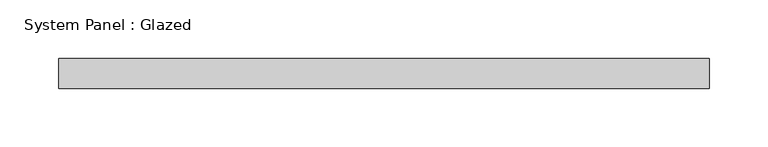
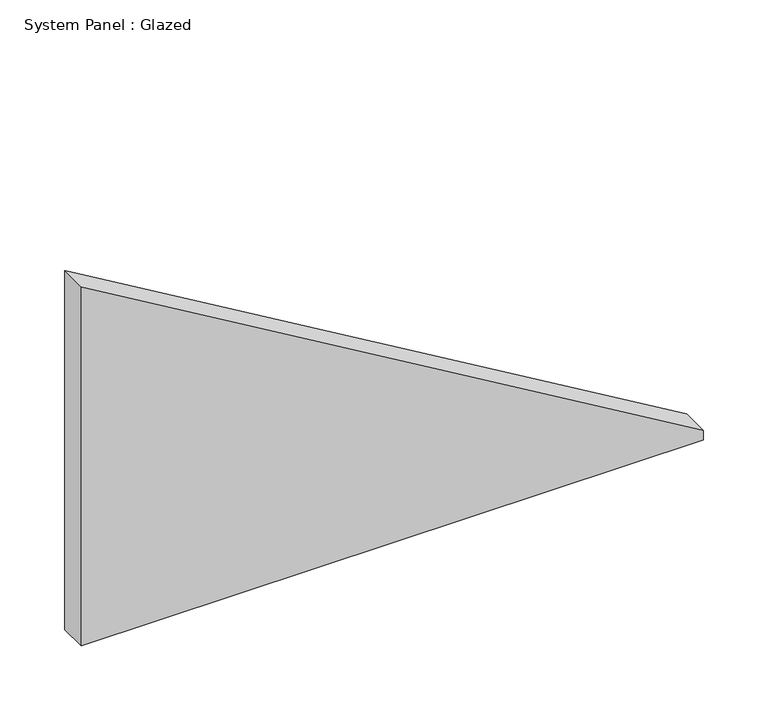
"""IFC4 building model written with IfcOpenShell, lengths in millimetres: plate geometry, System Panel : Glazed."""

from ifc_helpers import new_model, si_unit, frame, origin, place, context, project, spatial, polyline, outline, extrude, source, transform, mapped, element, save


def system_panel_glazed_02eac8f9(model_context):
    return source(origin(), model_context, "Body", "SweptSolid", [
        extrude(outline(polyline([(0.0, -276.6832607), (0.0, 276.6832607), (9.1085487, 276.6832607), (337.9987292, -276.6832607), (0.0, -276.6832607)])), frame((0.0, 19.05, 0.0), z_axis=(0.0, 1.0, 0.0), x_axis=(0.0, 0.0, 1.0)), (0.0, 0.0, 1.0), 25.4),
    ])


if __name__ == "__main__":
    model = new_model("IFC4")
    model_context = context("Model", 3, world=origin())
    ifc_project = project(units=[si_unit("LENGTHUNIT", "METRE", prefix="MILLI")], contexts=[model_context])
    site = spatial("IfcSite", under=ifc_project)
    building = spatial("IfcBuilding", under=site)
    placement = place(None, origin())
    system_panel_glazed_shape = system_panel_glazed_02eac8f9(model_context)
    element("IfcPlate", 1, ObjectType="System Panel : Glazed", at=placement, inside=building, context=model_context, shape_type="MappedRepresentation", body=[
        mapped(system_panel_glazed_shape, transform((0.0, 0.0, 0.0), x_axis=(1.0, 0.0, 0.0), y_axis=(0.0, 1.0, 0.0), z_axis=(0.0, 0.0, 1.0))),
    ])
    save(model, "model.ifc")

# Revit data of these elements
# Type "System Panel : Glazed"
#   Construction Type Id = "GSP4R"
#   Analytic Construction = "1/8 in Pilkington single glazing"
#   Visual Light Transmittance = 0.9
#   Solar Heat Gain Coefficient = 0.86
#   Heat Transfer Coefficient (U) = 1.18115 BTU/(h·ft²·°F)
#   Define Thermal Properties by = 1
# Element 1 (IfcPlate, "System Panel : Glazed")
#   Materials on its faces: "Glass"
# Materials
#   "Glass": class "Glass", colour RGB 0 128 192, transparency 0.75, Description = "Soda Lime Glass", Cost = 0
